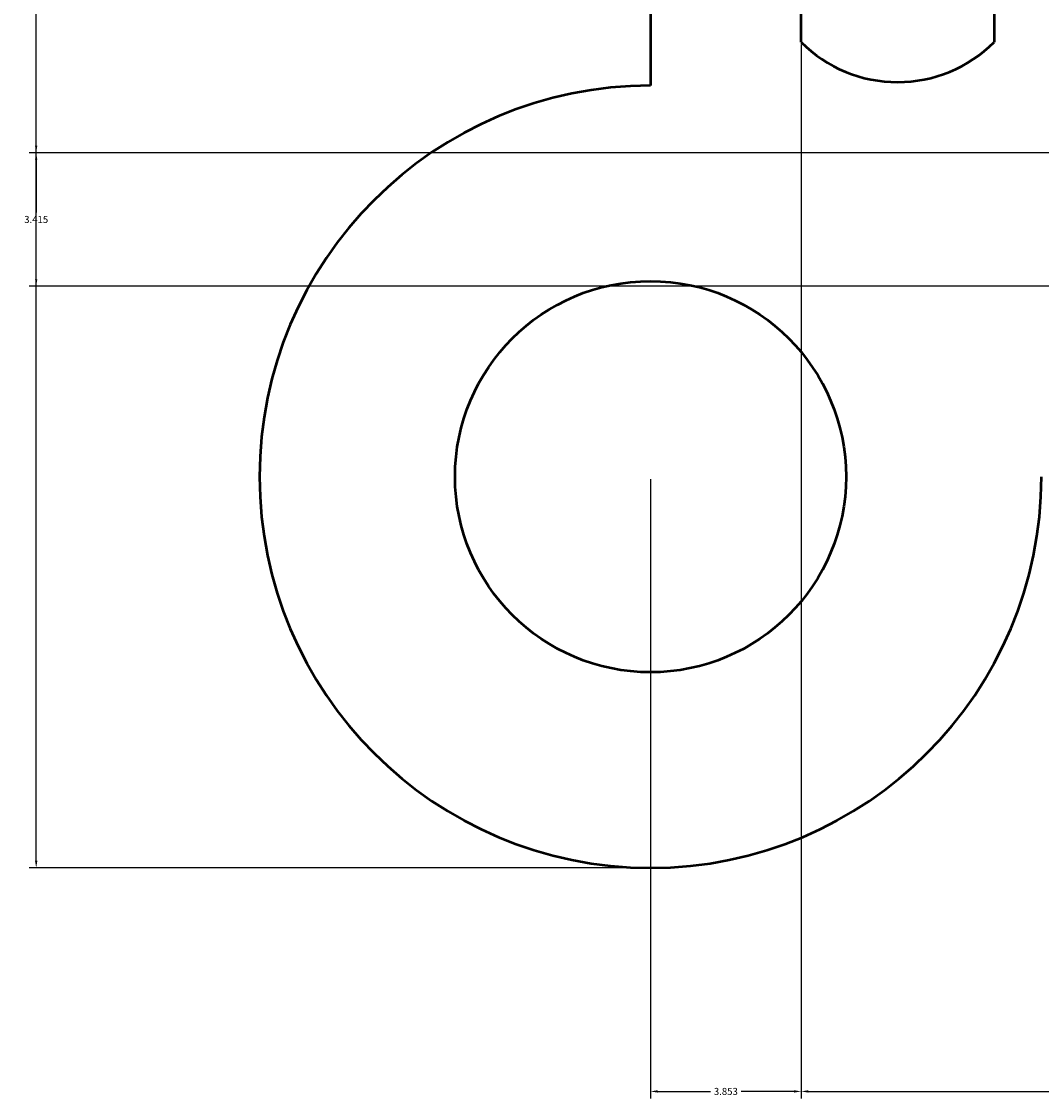
# Model space of a CAD drawing. Units: inches. Extents: x -14 to 108, y -9 to 83.
# Tile 1 of 13: x -14 to 12, y -9 to 19. Entities that reach past the tile are written whole.
import ezdxf

# ---------------------------------------------------------------- set-up
doc = ezdxf.new("R2010")
doc.units = ezdxf.units.IN
doc.header["$MEASUREMENT"] = 0
doc.layers.add('M-DIMS', color=2, linetype='Continuous', lineweight=18)
doc.layers.add('M-OUTL', color=7, linetype='Continuous', lineweight=50)
doc.styles.get("Standard").update_dxf_attribs({"font": 'arial.ttf'})
doc.dimstyles.get("Standard").update_dxf_attribs({"dimtxt": 0.18, "dimasz": 0.18, "dimexe": 0.18, "dimexo": 0.0625, "dimgap": 0.09, "dimtad": 0, "dimtih": 1, "dimtoh": 1, "dimzin": 0, "dimdsep": 46, "dimtxsty": 'Standard', "dimcen": 0.09, "dimadec": 0, "dimazin": 0, "dimtfac": 1, "dimtofl": 0, "dimtmove": 0, "dimatfit": 3, "dimfxl": 1, "dimtolj": 1, "dimtzin": 0, "dimarcsym": 0})

# ---------------------------------------------------------------- blocks, each defined once
blk = doc.blocks.new('SLOT-VERTICAL')
for points in [[(0, 1.021), (0, 40.458)], [(4.933, 40.458), (4.933, 1.021)]]:
    blk.add_lwpolyline(points)
blk.add_arc((2.466, 3.488), 3.489, 225, 315)
blk = doc.blocks.new('HOLE-D10')
blk.add_circle((5, 5), 5)
blk = doc.blocks.new('*D5')
at = {"layer": 'Defpoints', "color": 0, "transparency": 16777216}
for p in [(-13.617, 77.119), (2.098, 77.119), (2.098, -2.881)]:
    blk.add_point(p, dxfattribs=at)
at = {"layer": 'M-DIMS', "color": 0, "lineweight": -2, "transparency": 16777216}
for p, q in [((2.035, 77.119), (-13.797, 77.119)), ((-13.617, 76.939), (-13.617, 37.301)), ((-13.617, -2.701), (-13.617, 36.937)), ((2.035, -2.881), (-13.797, -2.881))]:
    blk.add_line(p, q, dxfattribs=at)
at = {"layer": 'M-DIMS', "color": 0, "transparency": 16777216}
for points in [[(-13.647, 76.939), (-13.587, 76.939), (-13.617, 77.119)], [(-13.647, -2.701), (-13.587, -2.701), (-13.617, -2.881)]]:
    blk.add_solid(points, dxfattribs=at)
at = {"layer": 'M-DIMS', "color": 0, "transparency": 16777216, "insert": (-13.617, 37.119), "char_height": 0.18, "attachment_point": 5}
blk.add_mtext('\\A1;80', dxfattribs=at)
blk = doc.blocks.new('*D6')
at = {"layer": 'Defpoints', "color": 0, "transparency": 16777216}
for p in [(5.951, 18.227), (2.098, 7.119), (5.951, -8.596)]:
    blk.add_point(p, dxfattribs=at)
at = {"layer": 'M-DIMS', "color": 0, "lineweight": -2, "transparency": 16777216}
for p, q in [((5.951, 18.165), (5.951, -8.776)), ((2.098, 7.057), (2.098, -8.776)), ((2.278, -8.596), (3.631, -8.596)), ((5.771, -8.596), (4.418, -8.596))]:
    blk.add_line(p, q, dxfattribs=at)
at = {"layer": 'M-DIMS', "color": 0, "transparency": 16777216}
for points in [[(2.278, -8.566), (2.278, -8.626), (2.098, -8.596)], [(5.771, -8.566), (5.771, -8.626), (5.951, -8.596)]]:
    blk.add_solid(points, dxfattribs=at)
at = {"layer": 'M-DIMS', "color": 0, "transparency": 16777216, "insert": (4.024, -8.596), "char_height": 0.18, "attachment_point": 5}
blk.add_mtext('\\A1;3.853', dxfattribs=at)
blk = doc.blocks.new('*D7')
at = {"layer": 'Defpoints', "color": 0, "transparency": 16777216}
for p in [(47.098, 37.119), (5.951, 18.227), (47.098, -8.596)]:
    blk.add_point(p, dxfattribs=at)
at = {"layer": 'M-DIMS', "color": 0, "lineweight": -2, "transparency": 16777216}
for p, q in [((47.098, 37.057), (47.098, -8.776)), ((5.951, 18.165), (5.951, -8.776)), ((6.131, -8.596), (26.126, -8.596)), ((46.918, -8.596), (26.922, -8.596))]:
    blk.add_line(p, q, dxfattribs=at)
at = {"layer": 'M-DIMS', "color": 0, "transparency": 16777216}
for points in [[(6.131, -8.566), (6.131, -8.626), (5.951, -8.596)], [(46.918, -8.566), (46.918, -8.626), (47.098, -8.596)]]:
    blk.add_solid(points, dxfattribs=at)
at = {"layer": 'M-DIMS', "color": 0, "transparency": 16777216, "insert": (26.524, -8.596), "char_height": 0.18, "attachment_point": 5}
blk.add_mtext('\\A1;41.15', dxfattribs=at)
blk = doc.blocks.new('*D19')
at = {"layer": 'Defpoints', "color": 0, "transparency": 16777216}
for p in [(-13.617, 37.119), (16.928, 37.119), (27.381, 15.402)]:
    blk.add_point(p, dxfattribs=at)
at = {"layer": 'M-DIMS', "color": 0, "lineweight": -2, "transparency": 16777216}
for p, q in [((16.865, 37.119), (-13.797, 37.119)), ((-13.617, 36.939), (-13.617, 26.441)), ((-13.617, 15.582), (-13.617, 26.08)), ((27.318, 15.402), (-13.797, 15.402))]:
    blk.add_line(p, q, dxfattribs=at)
at = {"layer": 'M-DIMS', "color": 0, "transparency": 16777216}
for points in [[(-13.647, 36.939), (-13.587, 36.939), (-13.617, 37.119)], [(-13.647, 15.582), (-13.587, 15.582), (-13.617, 15.402)]]:
    blk.add_solid(points, dxfattribs=at)
at = {"layer": 'M-DIMS', "color": 0, "transparency": 16777216, "insert": (-13.617, 26.261), "char_height": 0.18, "attachment_point": 5}
blk.add_mtext('\\A1;21.717', dxfattribs=at)
blk = doc.blocks.new('*D20')
at = {"layer": 'Defpoints', "color": 0, "transparency": 16777216}
for p in [(-13.617, 15.402), (27.381, 15.402), (46.1, 11.987)]:
    blk.add_point(p, dxfattribs=at)
at = {"layer": 'M-DIMS', "color": 0, "lineweight": -2, "transparency": 16777216}
for p, q in [((27.318, 15.402), (-13.797, 15.402)), ((-13.617, 15.222), (-13.617, 13.877)), ((-13.617, 12.167), (-13.617, 13.513)), ((46.038, 11.987), (-13.797, 11.987))]:
    blk.add_line(p, q, dxfattribs=at)
at = {"layer": 'M-DIMS', "color": 0, "transparency": 16777216}
for points in [[(-13.647, 15.222), (-13.587, 15.222), (-13.617, 15.402)], [(-13.647, 12.167), (-13.587, 12.167), (-13.617, 11.987)]]:
    blk.add_solid(points, dxfattribs=at)
at = {"layer": 'M-DIMS', "color": 0, "transparency": 16777216, "insert": (-13.617, 13.695), "char_height": 0.18, "attachment_point": 5}
blk.add_mtext('\\A1;3.415', dxfattribs=at)

msp = doc.modelspace()

# ---------------------------------------------------------------- linework, layer by layer
at = {"layer": 'M-OUTL'}
msp.add_lwpolyline([(2.0979, 57.1193), (2.0979, 17.1193)], dxfattribs=at)
msp.add_arc((2.0979, 7.1193), 10, 90, 0, dxfattribs=at)

# ---------------------------------------------------------------- block references
for name, p in [('SLOT-VERTICAL', (5.9511, 17.206)), ('HOLE-D10', (-2.902, 2.119))]:
    msp.add_blockref(name, p, dxfattribs=at)

# ---------------------------------------------------------------- dimensions: what is measured, and where the dimension line sits
at = {"layer": 'M-DIMS'}
for base, p1, p2, override, picture, middle in [((-13.6171, 77.1193), (2.0979, -2.8807), (2.0979, 77.1193), {"dimdec": 0, "dimlfac": 1, "dimrnd": 0, "dimzin": 0, "dimdsep": 46, "dimlunit": 2}, '*D5', (-13.6171, 37.1193)), ((-13.6171, 37.1193), (27.3809, 15.4023), (16.9278, 37.1193), {"dimdec": 3, "dimlfac": 1, "dimrnd": 0, "dimzin": 0, "dimdsep": 46, "dimlunit": 2}, '*D19', (-13.6171, 26.2608)), ((-13.6171, 15.4023), (46.1003, 11.987), (27.3809, 15.4023), {"dimdec": 3, "dimlfac": 1, "dimrnd": 0, "dimzin": 0, "dimdsep": 46, "dimlunit": 2}, '*D20', (-13.6171, 13.6947))]:
    dim = msp.add_linear_dim(base=base, p1=p1, p2=p2, angle=90, dimstyle='Standard', override=override, dxfattribs=at)
    dim.commit()
    dim.dimension.update_dxf_attribs({"geometry": picture, "text_midpoint": middle})
for base, p1, p2, override, picture, middle in [((47.0979, -8.5957), (5.9508, 18.2274), (47.0979, 37.1193), {"dimdec": 2, "dimlfac": 1, "dimrnd": 0, "dimzin": 0, "dimdsep": 46, "dimlunit": 2}, '*D7', (26.5244, -8.5957)), ((5.9508, -8.5957), (2.0979, 7.1193), (5.9508, 18.2274), {"dimdec": 3, "dimlfac": 1, "dimrnd": 0, "dimzin": 0, "dimdsep": 46, "dimlunit": 2}, '*D6', (4.0244, -8.5957))]:
    dim = msp.add_linear_dim(base=base, p1=p1, p2=p2, dimstyle='Standard', override=override, dxfattribs=at)
    dim.commit()
    dim.dimension.update_dxf_attribs({"geometry": picture, "text_midpoint": middle})

doc.saveas('drawing.dxf')
